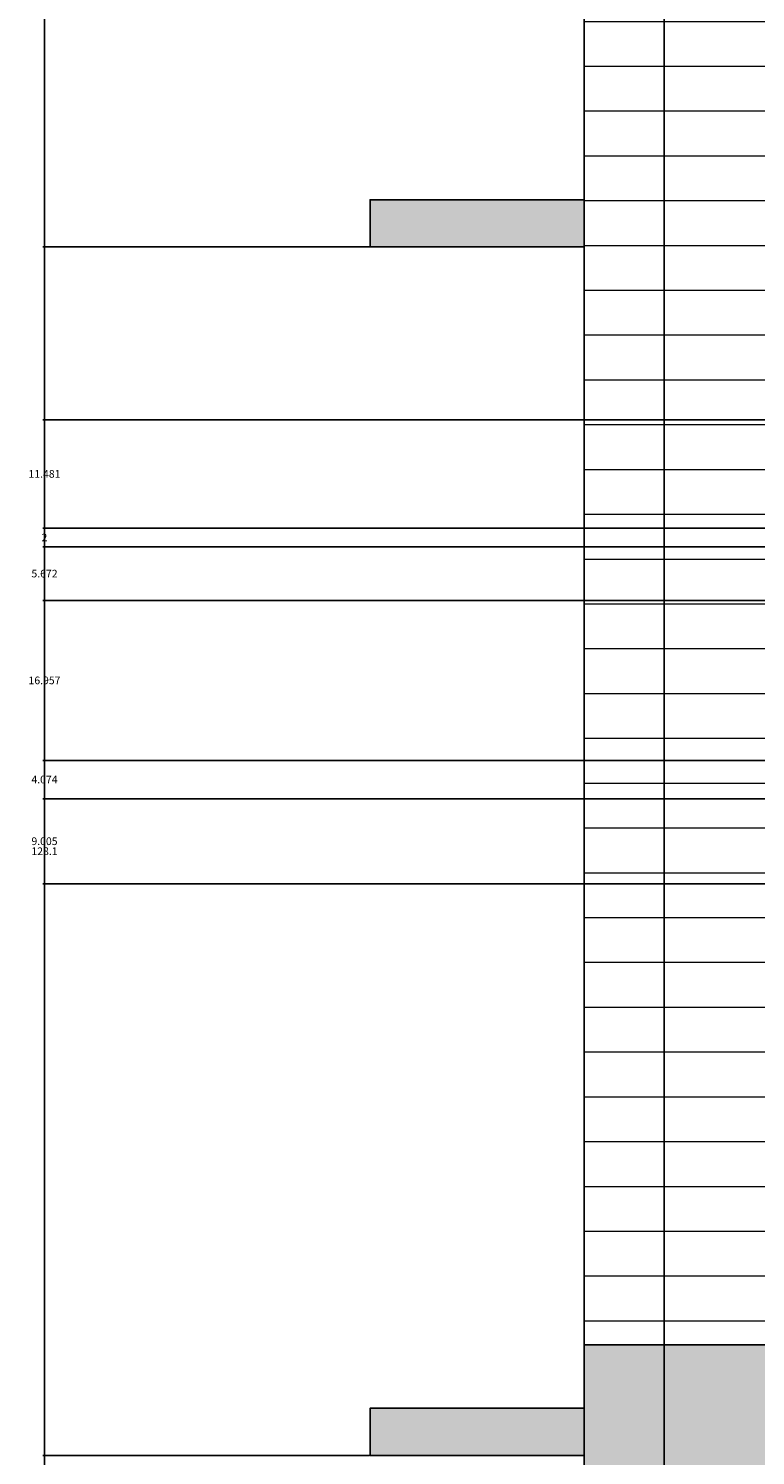
# Model space of a CAD drawing. Units: inches. Extents: x 36 to 594, y 79 to 831.
# Tile 7 of 30: x 36 to 113, y 294 to 446. Entities that reach past the tile are written whole.
import ezdxf

# ---------------------------------------------------------------- set-up
doc = ezdxf.new("R2010")
doc.units = ezdxf.units.IN
doc.header["$MEASUREMENT"] = 0
for name, color, linetype, lineweight in [('A-ANNO-DIMS', 2, 'Continuous', 18), ('A-ELEV', 7, 'Continuous', 25), ('A-ELEV-PATT', 8, 'Continuous', 13)]:
    doc.layers.add(name, color=color, linetype=linetype, lineweight=lineweight)
doc.styles.get("Standard").update_dxf_attribs({"font": 'arial.ttf'})
doc.dimstyles.get("Standard").update_dxf_attribs({"dimtxt": 0.8125, "dimasz": 0.18, "dimexe": 0.18, "dimexo": 0.0625, "dimgap": 0.09, "dimtad": 0, "dimtih": 1, "dimtoh": 1, "dimdec": 4, "dimzin": 0, "dimdsep": 46, "dimlunit": 4, "dimtxsty": 'Standard', "dimcen": 0.09, "dimadec": 0, "dimazin": 0, "dimtfac": 1, "dimtdec": 4, "dimtofl": 0, "dimtmove": 0, "dimatfit": 3, "dimfxl": 1, "dimtolj": 1, "dimtzin": 0, "dimarcsym": 0})

# ---------------------------------------------------------------- blocks, each defined once
blk = doc.blocks.new('*D28')
at = {"layer": 'A-ANNO-DIMS', "color": 0, "lineweight": -2, "transparency": 16777216}
for p, q in [((269.3, 796.05), (37.49, 796.05)), ((37.67, 795.87), (37.67, 455.63)), ((37.67, 114.39), (37.67, 454.62)), ((94.8, 114.21), (37.49, 114.21))]:
    blk.add_line(p, q, dxfattribs=at)
at = {"layer": 'A-ANNO-DIMS', "color": 0, "transparency": 16777216}
for points in [[(37.64, 795.87), (37.7, 795.87), (37.67, 796.05)], [(37.64, 114.39), (37.7, 114.39), (37.67, 114.21)]]:
    blk.add_solid(points, dxfattribs=at)
at = {"layer": 'Defpoints', "color": 0, "transparency": 16777216}
for p in [(37.67, 796.05), (269.36, 796.05), (94.87, 114.21)]:
    blk.add_point(p, dxfattribs=at)
at = {"layer": 'A-ANNO-DIMS', "color": 0, "transparency": 16777216, "insert": (37.67, 455.13), "char_height": 0.812, "attachment_point": 5}
blk.add_mtext('\\A1;681.8', dxfattribs=at)
blk = doc.blocks.new('*D43')
at = {"layer": 'A-ANNO-DIMS', "color": 0, "lineweight": -2, "transparency": 16777216}
for p, q in [((72.11, 422.59), (37.49, 422.59)), ((37.67, 422.41), (37.67, 359.04)), ((37.67, 294.66), (37.67, 358.03)), ((72.11, 294.48), (37.49, 294.48))]:
    blk.add_line(p, q, dxfattribs=at)
at = {"layer": 'A-ANNO-DIMS', "color": 0, "transparency": 16777216}
for points in [[(37.64, 422.41), (37.7, 422.41), (37.67, 422.59)], [(37.64, 294.66), (37.7, 294.66), (37.67, 294.48)]]:
    blk.add_solid(points, dxfattribs=at)
at = {"layer": 'Defpoints', "color": 0, "transparency": 16777216}
for p in [(37.67, 422.59), (72.17, 422.59), (72.17, 294.48)]:
    blk.add_point(p, dxfattribs=at)
at = {"layer": 'A-ANNO-DIMS', "color": 0, "transparency": 16777216, "insert": (37.67, 358.53), "char_height": 0.812, "attachment_point": 5}
blk.add_mtext('\\A1;128.1', dxfattribs=at)
blk = doc.blocks.new('*D44')
at = {"layer": 'A-ANNO-DIMS', "color": 0, "lineweight": -2, "transparency": 16777216}
for p, q in [((72.11, 603.6), (37.49, 603.6)), ((37.67, 603.42), (37.67, 513.6)), ((37.67, 422.77), (37.67, 512.59)), ((72.11, 422.59), (37.49, 422.59))]:
    blk.add_line(p, q, dxfattribs=at)
at = {"layer": 'A-ANNO-DIMS', "color": 0, "transparency": 16777216}
for points in [[(37.64, 603.42), (37.7, 603.42), (37.67, 603.6)], [(37.64, 422.77), (37.7, 422.77), (37.67, 422.59)]]:
    blk.add_solid(points, dxfattribs=at)
at = {"layer": 'Defpoints', "color": 0, "transparency": 16777216}
for p in [(37.67, 603.6), (72.17, 603.6), (72.17, 422.59)]:
    blk.add_point(p, dxfattribs=at)
at = {"layer": 'A-ANNO-DIMS', "color": 0, "transparency": 16777216, "insert": (37.67, 513.09), "char_height": 0.812, "attachment_point": 5}
blk.add_mtext('\\A1;181', dxfattribs=at)
blk = doc.blocks.new('*D60')
at = {"layer": 'A-ANNO-DIMS', "color": 0, "lineweight": -2, "transparency": 16777216}
for p, q in [((103.34, 286.24), (103.34, 830.73)), ((103.52, 830.55), (128.41, 830.55)), ((156.23, 830.55), (131.33, 830.55)), ((156.41, 264.68), (156.41, 830.73))]:
    blk.add_line(p, q, dxfattribs=at)
at = {"layer": 'A-ANNO-DIMS', "color": 0, "transparency": 16777216}
for points in [[(103.52, 830.58), (103.52, 830.52), (103.34, 830.55)], [(156.23, 830.58), (156.23, 830.52), (156.41, 830.55)]]:
    blk.add_solid(points, dxfattribs=at)
at = {"layer": 'Defpoints', "color": 0, "transparency": 16777216}
for p in [(156.41, 830.55), (103.34, 286.18), (156.41, 264.62)]:
    blk.add_point(p, dxfattribs=at)
at = {"layer": 'A-ANNO-DIMS', "color": 0, "transparency": 16777216, "insert": (129.87, 830.55), "char_height": 0.812, "attachment_point": 5}
blk.add_mtext('\\A1;53.07', dxfattribs=at)
blk = doc.blocks.new('*D111')
at = {"layer": 'A-ANNO-DIMS', "color": 0, "lineweight": -2, "transparency": 16777216}
for p, q in [((244.76, 364.09), (37.49, 364.09)), ((37.67, 363.91), (37.67, 360.09)), ((37.67, 355.26), (37.67, 359.08)), ((241.29, 355.08), (37.49, 355.08))]:
    blk.add_line(p, q, dxfattribs=at)
at = {"layer": 'A-ANNO-DIMS', "color": 0, "transparency": 16777216}
for points in [[(37.64, 363.91), (37.7, 363.91), (37.67, 364.09)], [(37.64, 355.26), (37.7, 355.26), (37.67, 355.08)]]:
    blk.add_solid(points, dxfattribs=at)
at = {"layer": 'Defpoints', "color": 0, "transparency": 16777216}
for p in [(37.67, 364.09), (244.82, 364.09), (241.36, 355.08)]:
    blk.add_point(p, dxfattribs=at)
at = {"layer": 'A-ANNO-DIMS', "color": 0, "transparency": 16777216, "insert": (37.67, 359.59), "char_height": 0.812, "attachment_point": 5}
blk.add_mtext('\\A1;9.005', dxfattribs=at)
blk = doc.blocks.new('*D112')
at = {"layer": 'A-ANNO-DIMS', "color": 0, "lineweight": -2, "transparency": 16777216}
for p, q in [((244.76, 368.16), (37.49, 368.16)), ((37.67, 367.98), (37.67, 366.63)), ((37.67, 364.27), (37.67, 365.62)), ((244.76, 364.09), (37.49, 364.09))]:
    blk.add_line(p, q, dxfattribs=at)
at = {"layer": 'A-ANNO-DIMS', "color": 0, "transparency": 16777216}
for points in [[(37.64, 367.98), (37.7, 367.98), (37.67, 368.16)], [(37.64, 364.27), (37.7, 364.27), (37.67, 364.09)]]:
    blk.add_solid(points, dxfattribs=at)
at = {"layer": 'Defpoints', "color": 0, "transparency": 16777216}
for p in [(37.67, 368.16), (244.82, 368.16), (244.82, 364.09)]:
    blk.add_point(p, dxfattribs=at)
at = {"layer": 'A-ANNO-DIMS', "color": 0, "transparency": 16777216, "insert": (37.67, 366.13), "char_height": 0.812, "attachment_point": 5}
blk.add_mtext('\\A1;4.074', dxfattribs=at)
blk = doc.blocks.new('*D113')
at = {"layer": 'A-ANNO-DIMS', "color": 0, "lineweight": -2, "transparency": 16777216}
for p, q in [((244.76, 385.12), (37.49, 385.12)), ((37.67, 384.94), (37.67, 377.15)), ((37.67, 368.34), (37.67, 376.14)), ((244.76, 368.16), (37.49, 368.16))]:
    blk.add_line(p, q, dxfattribs=at)
at = {"layer": 'A-ANNO-DIMS', "color": 0, "transparency": 16777216}
for points in [[(37.64, 384.94), (37.7, 384.94), (37.67, 385.12)], [(37.64, 368.34), (37.7, 368.34), (37.67, 368.16)]]:
    blk.add_solid(points, dxfattribs=at)
at = {"layer": 'Defpoints', "color": 0, "transparency": 16777216}
for p in [(37.67, 385.12), (244.82, 385.12), (244.82, 368.16)]:
    blk.add_point(p, dxfattribs=at)
at = {"layer": 'A-ANNO-DIMS', "color": 0, "transparency": 16777216, "insert": (37.67, 376.64), "char_height": 0.812, "attachment_point": 5}
blk.add_mtext('\\A1;16.957', dxfattribs=at)
blk = doc.blocks.new('*D114')
at = {"layer": 'A-ANNO-DIMS', "color": 0, "lineweight": -2, "transparency": 16777216}
for p, q in [((241.29, 390.79), (37.49, 390.79)), ((37.67, 390.61), (37.67, 388.46)), ((37.67, 385.3), (37.67, 387.45)), ((244.76, 385.12), (37.49, 385.12))]:
    blk.add_line(p, q, dxfattribs=at)
at = {"layer": 'A-ANNO-DIMS', "color": 0, "transparency": 16777216}
for points in [[(37.64, 390.61), (37.7, 390.61), (37.67, 390.79)], [(37.64, 385.3), (37.7, 385.3), (37.67, 385.12)]]:
    blk.add_solid(points, dxfattribs=at)
at = {"layer": 'Defpoints', "color": 0, "transparency": 16777216}
for p in [(37.67, 390.79), (241.36, 390.79), (244.82, 385.12)]:
    blk.add_point(p, dxfattribs=at)
at = {"layer": 'A-ANNO-DIMS', "color": 0, "transparency": 16777216, "insert": (37.67, 387.96), "char_height": 0.812, "attachment_point": 5}
blk.add_mtext('\\A1;5.672', dxfattribs=at)
blk = doc.blocks.new('*D115')
at = {"layer": 'A-ANNO-DIMS', "color": 0, "lineweight": -2, "transparency": 16777216}
for p, q in [((241.29, 392.79), (37.49, 392.79)), ((37.67, 392.61), (37.67, 392.29)), ((241.29, 390.79), (37.49, 390.79)), ((37.67, 390.97), (37.67, 391.29))]:
    blk.add_line(p, q, dxfattribs=at)
at = {"layer": 'A-ANNO-DIMS', "color": 0, "transparency": 16777216}
for points in [[(37.64, 392.61), (37.7, 392.61), (37.67, 392.79)], [(37.64, 390.97), (37.7, 390.97), (37.67, 390.79)]]:
    blk.add_solid(points, dxfattribs=at)
at = {"layer": 'Defpoints', "color": 0, "transparency": 16777216}
for p in [(37.67, 392.79), (241.36, 392.79), (241.36, 390.79)]:
    blk.add_point(p, dxfattribs=at)
at = {"layer": 'A-ANNO-DIMS', "color": 0, "transparency": 16777216, "insert": (37.67, 391.79), "char_height": 0.812, "attachment_point": 5}
blk.add_mtext('\\A1;2', dxfattribs=at)
blk = doc.blocks.new('*D116')
at = {"layer": 'A-ANNO-DIMS', "color": 0, "lineweight": -2, "transparency": 16777216}
for p, q in [((241.29, 404.27), (37.49, 404.27)), ((37.67, 404.09), (37.67, 399.04)), ((37.67, 392.97), (37.67, 398.03)), ((241.29, 392.79), (37.49, 392.79))]:
    blk.add_line(p, q, dxfattribs=at)
at = {"layer": 'A-ANNO-DIMS', "color": 0, "transparency": 16777216}
for points in [[(37.64, 404.09), (37.7, 404.09), (37.67, 404.27)], [(37.64, 392.97), (37.7, 392.97), (37.67, 392.79)]]:
    blk.add_solid(points, dxfattribs=at)
at = {"layer": 'Defpoints', "color": 0, "transparency": 16777216}
for p in [(37.67, 404.27), (241.36, 404.27), (241.36, 392.79)]:
    blk.add_point(p, dxfattribs=at)
at = {"layer": 'A-ANNO-DIMS', "color": 0, "transparency": 16777216, "insert": (37.67, 398.53), "char_height": 0.812, "attachment_point": 5}
blk.add_mtext('\\A1;11.481', dxfattribs=at)

msp = doc.modelspace()

# ---------------------------------------------------------------- hatches: boundary and pattern name
at = {"layer": 'A-ELEV-PATT'}
h = msp.add_hatch(color=256, dxfattribs=at)
h.dxf.hatch_style = 1
h.paths.add_polyline_path([(398.0873, 796.0465), (269.3592, 796.0465), (269.3592, 770.1455), (397.8159, 770.1455)])
h.paths.add_polyline_path([(397.7518, 764.0341), (269.3592, 764.0341), (269.3592, 630.0394), (341.8367, 630.0394), (341.8367, 720.595), (335.0881, 728.3699), (329.982, 735.3373), (345.3661, 727.7743), (397.1052, 702.3389)])
h.paths.add_polyline_path([(341.8367, 594.2124), (201.4189, 594.2124), (201.4189, 475.4136), (232.8216, 475.4136), (232.8216, 524.6037), (341.8367, 524.6037)])
h.paths.add_polyline_path([(177.525, 594.2124), (118.7598, 594.2124), (118.7598, 450.2124), (177.525, 450.2124)])
h.paths.add_polyline_path([(424.4958, 594.2124), (365.7306, 594.2124), (365.7306, 450.2124), (424.4958, 450.2124)])
h.paths.add_polyline_path([(241.3553, 404.2737), (355.8569, 404.2737), (355.8569, 355.0836), (424.5492, 355.0836), (424.5492, 425.7333), (118.7598, 426.2844), (118.7598, 355.0836), (241.3553, 355.0836)])
h.paths.add_polyline_path([(448.3898, 306.2124), (217.0273, 306.2124), (217.0273, 142.2124), (254.0293, 142.2124), (254.0293, 150.9347), (254.0293, 286.1802), (401.5491, 286.1802), (401.5491, 150.9347), (401.5491, 142.2124), (448.3898, 142.2124)])
h.paths.add_polyline_path([(448.3898, 142.2124), (401.5491, 142.2124), (217.0273, 142.2124), (217.0273, 114.2124), (448.3898, 114.2124)])
h.paths.add_polyline_path([(217.0273, 306.2124), (174.7353, 306.2124), (94.8658, 306.2124), (94.8658, 162.2124), (103.3368, 162.2124), (103.3368, 264.6224), (103.3368, 286.1802), (217.0273, 286.1802)])
h = msp.add_hatch(color=256, dxfattribs=at)
h.dxf.hatch_style = 1
h.paths.add_polyline_path([(94.8658, 608.6081), (72.1733, 608.6081), (72.1733, 603.598), (94.8658, 603.598)])
h.paths.add_polyline_path([(94.8658, 427.5982), (72.1733, 427.5982), (72.1733, 422.5882), (94.8658, 422.5882)])
h.paths.add_polyline_path([(94.8658, 299.486), (72.1733, 299.486), (72.1733, 294.4759), (94.8658, 294.4759)])
h.paths.add_polyline_path([(269.3592, 770.1455), (260.5727, 770.1455), (260.5727, 764.0341), (269.3592, 764.0341)])
h.paths.add_polyline_path([(410.2381, 770.1455), (269.3592, 770.1455), (269.3592, 764.0341), (410.2381, 764.0341)])
h = msp.add_hatch(dxfattribs=at)
h.set_pattern_fill('ANSI31', color=256, scale=38, angle=135)
h.paths.add_polyline_path([(448.3898, 450.2124), (94.8658, 450.2124), (94.8658, 306.2124), (174.7353, 306.2124), (448.3898, 306.2124), (448.3898, 367.5118)])
h.paths.add_polyline_path([(424.5492, 425.7333), (424.5492, 329.5325), (118.7598, 330.0836), (118.7598, 354.0836), (118.7598, 426.2844)], flags=16)
h.paths.add_polyline_path([(355.8569, 404.2737), (355.8569, 355.0836), (241.3553, 355.0836), (241.3553, 404.2737)], flags=0)
h.paths.add_polyline_path([(269.0393, 390.7924), (269.0393, 355.0836), (244.8248, 355.0836), (244.8248, 364.0887), (263.8892, 364.0887), (263.8892, 355.0836), (267.0393, 355.0836), (267.0393, 390.7924)], flags=0)
h.paths.add_polyline_path([(303.9765, 436.9126, -1), (313.1496, 436.9126, -1)], flags=16)
h.paths.add_polyline_path([(421.9473, 354.0836), (421.9376, 348.6883), (421.9376, 333.9204), (401.6342, 333.9204), (401.6705, 354.0836), (400.6705, 354.0836), (400.6608, 348.7267), (400.6608, 333.9587), (380.3574, 333.9587), (380.3937, 354.0836), (379.3937, 354.0836), (379.3841, 348.765), (379.3841, 333.997), (359.0807, 333.997), (359.1169, 354.0836), (358.1169, 354.0836), (358.1074, 348.8034), (358.1074, 334.0354), (337.804, 334.0354), (337.8401, 354.0836), (336.8401, 354.0836), (336.8306, 348.8417), (336.8306, 334.0737), (316.5272, 334.0737), (316.5633, 354.0836), (315.5633, 354.0836), (315.5539, 348.8801), (315.5539, 334.1121), (295.2505, 334.1121), (295.2865, 354.0836), (294.2865, 354.0836), (294.2772, 348.9184), (294.2772, 334.1504), (273.9738, 334.1504), (274.0097, 354.0836), (273.0097, 354.0836), (273.0005, 348.9568), (273.0005, 334.1888), (252.697, 334.1888), (252.7329, 354.0836), (251.7329, 354.0836), (251.7237, 348.9951), (251.7237, 334.2271), (231.4203, 334.2271), (231.4561, 354.0836), (230.4561, 354.0836), (230.447, 349.0335), (230.447, 334.2655), (210.1436, 334.2655), (210.1793, 354.0836), (209.1793, 354.0836), (209.1703, 349.0718), (209.1703, 334.3038), (188.8668, 334.3038), (188.9025, 354.0836), (187.9025, 354.0836), (187.8935, 349.1101), (187.8935, 334.3422), (167.5901, 334.3422), (167.6257, 354.0836), (166.6257, 354.0836), (166.6168, 349.1485), (166.6168, 334.3805), (146.3134, 334.3805), (146.3489, 354.0836), (145.3489, 354.0836), (145.3401, 349.1868), (145.3401, 334.4189), (125.0366, 334.4189), (125.0721, 354.0836)], flags=0)
h.paths.add_polyline_path([(266.285, 436.9126, -1), (275.458, 436.9126, -1)], flags=16)
h.paths.add_polyline_path([(367.0204, 316.8739, -1), (357.8474, 316.8739, -1)], flags=16)
h.paths.add_polyline_path([(347.6933, 316.8739, -1), (338.5202, 316.8739, -1)], flags=16)
h.paths.add_polyline_path([(329.574, 316.8739, -1), (320.401, 316.8739, -1)], flags=16)
h.paths.add_polyline_path([(263.8892, 385.1199), (263.8892, 368.1628), (244.8248, 368.1628), (244.8248, 385.1199)], flags=0)
h.paths.add_polyline_path([(216.2543, 436.9126, -1), (225.4274, 436.9126, -1)], flags=16)
h.paths.add_polyline_path([(275.458, 316.8739, -1), (266.285, 316.8739, -1)], flags=16)
h.paths.add_polyline_path([(225.4274, 316.8739, -1), (216.2543, 316.8739, -1)], flags=16)

# ---------------------------------------------------------------- linework, layer by layer
at = {"layer": 'A-ELEV'}
for p, q in [((94.8658, 306.2124), (94.8658, 450.2124)), ((94.8658, 162.2124), (94.8658, 306.2124)), ((94.8658, 306.2124), (174.7353, 306.2124))]:
    msp.add_line(p, q, dxfattribs=at)
for points in [[(94.8658, 427.5982), (72.1733, 427.5982), (72.1733, 422.5882), (94.8658, 422.5882)], [(94.8658, 299.486), (72.1733, 299.486), (72.1733, 294.4759), (94.8658, 294.4759)]]:
    msp.add_lwpolyline(points, close=True, dxfattribs=at)

# ---------------------------------------------------------------- dimensions: what is measured, and where the dimension line sits
at = {"layer": 'A-ANNO-DIMS'}
dim = msp.add_linear_dim(base=(156.4069, 830.5465), p1=(103.3368, 286.1802), p2=(156.4069, 264.6224), dimstyle='Standard', override={"dimdec": 2, "dimlfac": 1, "dimrnd": 0, "dimzin": 0, "dimdsep": 46, "dimlunit": 2}, dxfattribs=at)
dim.commit()
dim.dimension.update_dxf_attribs({"geometry": '*D60', "text_midpoint": (129.8718, 830.5465)})
for base, p1, p2, override, picture, middle in [((37.6733, 796.0465), (94.8658, 114.2124), (269.3592, 796.0465), {"dimdec": 1, "dimlfac": 1, "dimrnd": 0, "dimzin": 0, "dimdsep": 46, "dimlunit": 2}, '*D28', (37.6733, 455.1294)), ((37.6733, 603.598), (72.1733, 422.5882), (72.1733, 603.598), {"dimdec": 0, "dimlfac": 1, "dimrnd": 0, "dimzin": 0, "dimdsep": 46, "dimlunit": 2}, '*D44', (37.6733, 513.0931)), ((37.6733, 422.5882), (72.1733, 294.4759), (72.1733, 422.5882), {"dimdec": 1, "dimlfac": 1, "dimrnd": 0, "dimzin": 0, "dimdsep": 46, "dimlunit": 2}, '*D43', (37.6733, 358.5321)), ((37.6733, 404.2737), (241.3553, 392.7924), (241.3553, 404.2737), {"dimdec": 3, "dimlfac": 1, "dimrnd": 0, "dimzin": 0, "dimdsep": 46, "dimlunit": 2}, '*D116', (37.6733, 398.533)), ((37.6733, 392.7924), (241.3553, 390.7924), (241.3553, 392.7924), {"dimdec": 0, "dimlfac": 1, "dimrnd": 0, "dimzin": 0, "dimdsep": 46, "dimlunit": 2}, '*D115', (37.6733, 391.7924)), ((37.67335, 390.79236), (244.82478, 385.11988), (241.3553, 390.79236), {"dimdec": 3, "dimlfac": 1, "dimrnd": 0, "dimzin": 0, "dimdsep": 46, "dimlunit": 2}, '*D114', (37.67335, 387.95612)), ((37.6733, 385.1199), (244.8248, 368.1628), (244.8248, 385.1199), {"dimdec": 3, "dimlfac": 1, "dimrnd": 0, "dimzin": 0, "dimdsep": 46, "dimlunit": 2}, '*D113', (37.6733, 376.6414)), ((37.6733, 368.1628), (244.8248, 364.0887), (244.8248, 368.1628), {"dimdec": 3, "dimlfac": 1, "dimrnd": 0, "dimzin": 0, "dimdsep": 46, "dimlunit": 2}, '*D112', (37.6733, 366.1258)), ((37.6733, 364.0887), (241.3553, 355.0836), (244.8248, 364.0887), {"dimdec": 3, "dimlfac": 1, "dimrnd": 0, "dimzin": 0, "dimdsep": 46, "dimlunit": 2}, '*D111', (37.6733, 359.5862))]:
    dim = msp.add_linear_dim(base=base, p1=p1, p2=p2, angle=90, dimstyle='Standard', override=override, dxfattribs=at)
    dim.commit()
    dim.dimension.update_dxf_attribs({"geometry": picture, "text_midpoint": middle})

doc.saveas('drawing.dxf')
